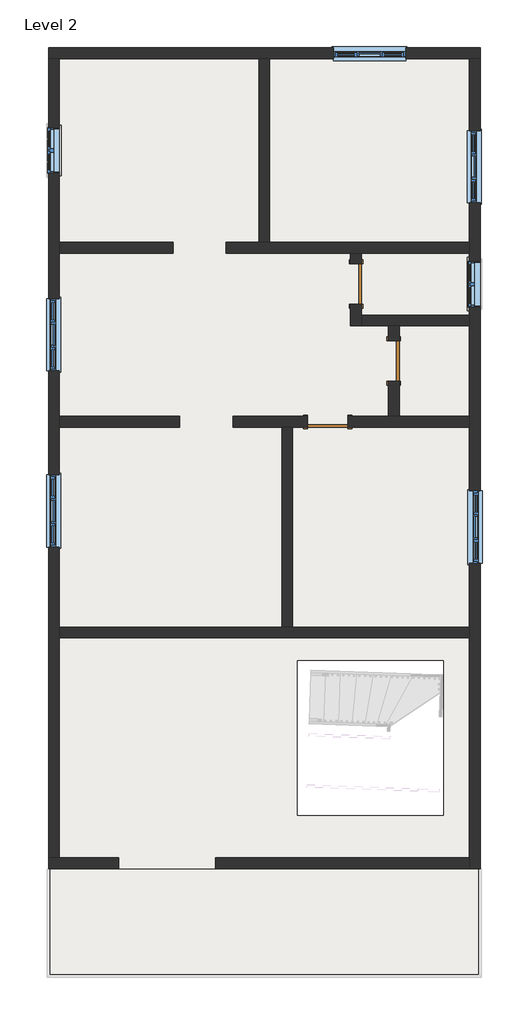
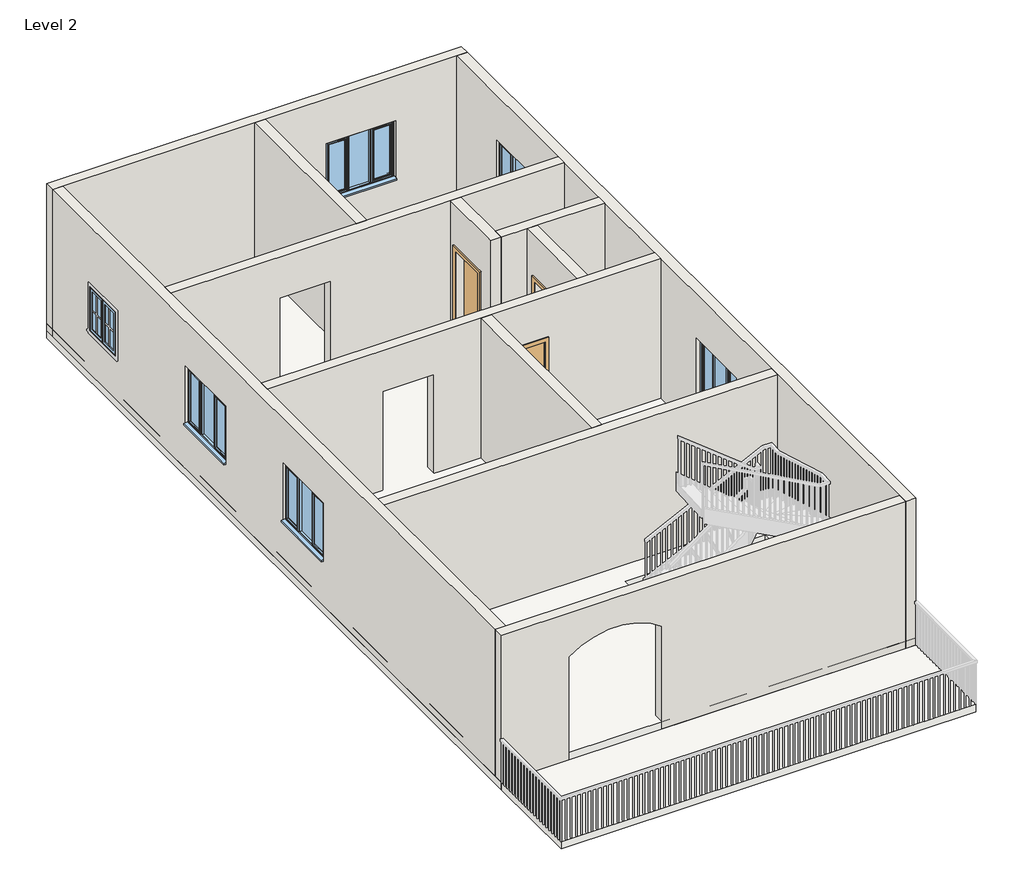
# One storey, part 1 of 3: 12 walls, 7 windows, 3 doors, 2 slabs, 1 roof.
"""IFC4 building model written with IfcOpenShell, lengths in millimetres."""

from ifc_helpers import new_model, si_unit, frame, origin, place, context, project, spatial, polyline, circle_curve, outline, extrude, faceted_brep, transform, mapped, element, save
from ifc_brep_helpers import plane_surface, revolved_surface, advanced_brep
from components import door_b6acaa4e, window_c29befe5, windows_tpl_plain_1360x1210mm_e2a6c9d8

model = new_model("IFC4")

# Units and contexts
model_context = context("Model", 3, world=origin())
ifc_project = project(units=[si_unit("LENGTHUNIT", "METRE", prefix="MILLI")], contexts=[model_context])

# Site, building, storey
site = spatial("IfcSite", under=ifc_project)
building = spatial("IfcBuilding", under=site)
storey = spatial("IfcBuildingStorey", under=building, Name="Level 2", Elevation=3048.0)

# Doors
placement = place(None, origin())
door_shape = door_b6acaa4e(model_context)
element("IfcDoor", 1, ObjectType="Single-Flush : 30\" x 84\"", at=placement, inside=storey, context=model_context, shape_type="MappedRepresentation", body=[
    mapped(door_shape, transform((-9158.3126504, 6947.728857, 3048.0), x_axis=(0.0, -1.0, 0.0), y_axis=(1.0, 0.0, 0.0), z_axis=(0.0, 0.0, 1.0))),
])
element("IfcDoor", 2, ObjectType="Single-Flush : 30\" x 84\"", at=placement, inside=storey, context=model_context, shape_type="MappedRepresentation", body=[
    mapped(door_shape, transform((-9691.7126504, 4356.928857, 3048.0), x_axis=(-1.0, 0.0, 0.0), y_axis=(0.0, -1.0, 0.0), z_axis=(0.0, 0.0, 1.0))),
])
element("IfcDoor", 3, ObjectType="Single-Flush : 30\" x 84\"", at=placement, inside=storey, context=model_context, shape_type="MappedRepresentation", body=[
    mapped(door_shape, transform((-8447.1126504, 5499.928857, 3048.0), x_axis=(0.0, -1.0, 0.0), y_axis=(1.0, 0.0, 0.0), z_axis=(0.0, 0.0, 1.0))),
])

# Roof
element("IfcRoof", 4, ObjectType="Generic - 12\"", at=placement, inside=storey, context=model_context, shape_type="SweptSolid", body=[
    extrude(outline(polyline([(-6821.5126504, 11392.728857), (-6821.5126504, -4050.471143), (-14949.5126504, -4050.471143), (-14949.5126504, 11392.728857), (-6821.5126504, 11392.728857)]), holes=[polyline([(-7518.4, -135.4836), (-10261.6, -135.4836), (-10261.6, -3048.381), (-7518.4, -3048.381), (-7518.4, -135.4836)])]), frame((0.0, 0.0, 3048.0), z_axis=(0.0, 0.0, 1.0), x_axis=(1.0, 0.0, 0.0)), (0.0, 0.0, 1.0), 152.4),
])

# Slabs
element("IfcSlab", 5, ObjectType="Generic - 12\"", at=placement, inside=storey, context=model_context, shape_type="SweptSolid", body=[
    extrude(outline(polyline([(-6821.5126504, 11392.728857), (-6821.5126504, -4050.471143), (-14949.5126504, -4050.471143), (-14949.5126504, 11392.728857), (-6821.5126504, 11392.728857)]), holes=[polyline([(-7518.4, -135.4836), (-10261.6, -135.4836), (-10261.6, -3048.381), (-7518.4, -3048.381), (-7518.4, -135.4836)])]), frame((0.0, 0.0, 2895.6), z_axis=(0.0, 0.0, 1.0), x_axis=(1.0, 0.0, 0.0)), (0.0, 0.0, 1.0), 152.4),
])
element("IfcSlab", 6, ObjectType="Generic - 12\"", at=placement, inside=storey, context=model_context, shape_type="SweptSolid", body=[
    extrude(outline(polyline([(-6821.5126504, -4050.471143), (-6821.5126504, -6082.471143), (-14949.5126504, -6082.471143), (-14949.5126504, -4050.471143), (-6821.5126504, -4050.471143)])), frame((0.0, 0.0, 2895.6), z_axis=(0.0, 0.0, 1.0), x_axis=(1.0, 0.0, 0.0)), (0.0, 0.0, 1.0), 152.4),
])

# Walls
element("IfcWall", 7, ObjectType="Generic - 4.5\" p", at=placement, inside=storey, context=model_context, shape_type="SweptSolid", body=[
    extrude(outline(polyline([(-10987.1126504, 7735.128857), (-10987.1126504, 11189.528857), (-10783.9126504, 11189.528857), (-10783.9126504, 7735.128857), (-10987.1126504, 7735.128857)])), frame((0.0, 0.0, 3048.0), z_axis=(0.0, 0.0, 1.0), x_axis=(1.0, 0.0, 0.0)), (0.0, 0.0, 1.0), 3048.0),
])
element("IfcWall", 8, ObjectType="Generic - 4.5\" p", at=placement, inside=storey, context=model_context, shape_type="Brep", body=[
    faceted_brep([(-7024.7126504, 7735.128857, 3048.0), (-10783.9126504, 7735.128857, 3048.0), (-10987.1126504, 7735.128857, 3048.0), (-11604.7126504, 7735.128857, 3048.0), (-11604.7126504, 7735.128857, 5248.0), (-12604.7126504, 7735.128857, 5248.0), (-12604.7126504, 7735.128857, 3048.0), (-14746.3126504, 7735.128857, 3048.0), (-14746.3126504, 7735.128857, 6096.0), (-10987.1126504, 7735.128857, 6096.0), (-10783.9126504, 7735.128857, 6096.0), (-7024.7126504, 7735.128857, 6096.0), (-11604.7126504, 7531.928857, 5248.0), (-11604.7126504, 7531.928857, 3048.0), (-9259.9126504, 7531.928857, 3048.0), (-9056.7126504, 7531.928857, 3048.0), (-7024.7126504, 7531.928857, 3048.0), (-7024.7126504, 7531.928857, 6096.0), (-9056.7126504, 7531.928857, 6096.0), (-9259.9126504, 7531.928857, 6096.0), (-14746.3126504, 7531.928857, 6096.0), (-14746.3126504, 7531.928857, 3048.0), (-12604.7126504, 7531.928857, 3048.0), (-12604.7126504, 7531.928857, 5248.0)], [[[0, 1, 2, 3, 4, 5, 6, 7, 8, 9, 10, 11]], [[12, 13, 14, 15, 16, 17, 18, 19, 20, 21, 22, 23]], [[22, 21, 7, 6]], [[16, 15, 14, 13, 3, 2, 1, 0]], [[11, 10, 9, 8, 20, 19, 18, 17]], [[8, 7, 21, 20]], [[0, 11, 17, 16]], [[4, 3, 13, 12]], [[5, 4, 12, 23]], [[6, 5, 23, 22]]]),
])
element("IfcWall", 9, ObjectType="Generic - 4.5\" p", at=placement, inside=storey, context=model_context, shape_type="Brep", body=[
    faceted_brep([(-9259.9126504, 6566.728857, 5181.6), (-9259.9126504, 6566.728857, 3048.0), (-9259.9126504, 6160.328857, 3048.0), (-9259.9126504, 6160.328857, 6096.0), (-9259.9126504, 7531.928857, 6096.0), (-9259.9126504, 7531.928857, 3048.0), (-9259.9126504, 7328.728857, 3048.0), (-9259.9126504, 7328.728857, 5181.6), (-9056.7126504, 6160.328857, 3048.0), (-9056.7126504, 6363.528857, 3048.0), (-9056.7126504, 6566.728857, 3048.0), (-9056.7126504, 6566.728857, 5181.6), (-9056.7126504, 7328.728857, 5181.6), (-9056.7126504, 7328.728857, 3048.0), (-9056.7126504, 7531.928857, 3048.0), (-9056.7126504, 7531.928857, 6096.0), (-9056.7126504, 6363.528857, 6096.0), (-9056.7126504, 6160.328857, 6096.0)], [[[0, 1, 2, 3, 4, 5, 6, 7]], [[8, 9, 10, 11, 12, 13, 14, 15, 16, 17]], [[6, 5, 14, 13]], [[2, 1, 10, 9, 8]], [[4, 3, 17, 16, 15]], [[5, 4, 15, 14]], [[3, 2, 8, 17]], [[11, 10, 1, 0]], [[12, 11, 0, 7]], [[13, 12, 7, 6]]]),
])
element("IfcWall", 10, ObjectType="Generic - 4.5\" p", at=placement, inside=storey, context=model_context, shape_type="Brep", body=[
    faceted_brep([(-9056.7126504, 6160.328857, 3048.0), (-8548.7126504, 6160.328857, 3048.0), (-8345.5126504, 6160.328857, 3048.0), (-7024.7126504, 6160.328857, 3048.0), (-7024.7126504, 6160.328857, 6096.0), (-8345.5126504, 6160.328857, 6096.0), (-8548.7126504, 6160.328857, 6096.0), (-9056.7126504, 6160.328857, 6096.0), (-9056.7126504, 6363.528857, 3048.0), (-9056.7126504, 6363.528857, 6096.0), (-7024.7126504, 6363.528857, 6096.0), (-7024.7126504, 6363.528857, 3048.0)], [[[0, 1, 2, 3, 4, 5, 6, 7]], [[8, 9, 10, 11]], [[3, 2, 1, 0, 8, 11]], [[7, 6, 5, 4, 10, 9]], [[0, 7, 9, 8]], [[4, 3, 11, 10]]]),
])
element("IfcWall", 11, ObjectType="Generic - 4.5\" p", at=placement, inside=storey, context=model_context, shape_type="SweptSolid", body=[
    extrude(outline(polyline([(5118.928857, 5181.6), (5118.928857, 3048.0), (4458.528857, 3048.0), (4458.528857, 6096.0), (6160.328857, 6096.0), (6160.328857, 3048.0), (5880.928857, 3048.0), (5880.928857, 5181.6), (5118.928857, 5181.6)])), frame((-8548.7126504, 0.0, 0.0), z_axis=(1.0, 0.0, 0.0), x_axis=(0.0, 1.0, 0.0)), (0.0, 0.0, 1.0), 203.2),
])
element("IfcWall", 12, ObjectType="Generic - 4.5\" p", at=placement, inside=storey, context=model_context, shape_type="Brep", body=[
    faceted_brep([(-10072.7126504, 4458.528857, 5181.6), (-10072.7126504, 4458.528857, 3048.0), (-11477.7126504, 4458.528857, 3048.0), (-11477.7126504, 4458.528857, 5248.0), (-12477.7126504, 4458.528857, 5248.0), (-12477.7126504, 4458.528857, 3048.0), (-14746.3126504, 4458.528857, 3048.0), (-14746.3126504, 4458.528857, 6096.0), (-8548.7126504, 4458.528857, 6096.0), (-8345.5126504, 4458.528857, 6096.0), (-7024.7126504, 4458.528857, 6096.0), (-7024.7126504, 4458.528857, 3048.0), (-8345.5126504, 4458.528857, 3048.0), (-8548.7126504, 4458.528857, 3048.0), (-9310.7126504, 4458.528857, 3048.0), (-9310.7126504, 4458.528857, 5181.6), (-11477.7126504, 4255.328857, 3048.0), (-10555.3126504, 4255.328857, 3048.0), (-10352.1126504, 4255.328857, 3048.0), (-10072.7126504, 4255.328857, 3048.0), (-10072.7126504, 4255.328857, 5181.6), (-9310.7126504, 4255.328857, 5181.6), (-9310.7126504, 4255.328857, 3048.0), (-7024.7126504, 4255.328857, 3048.0), (-7024.7126504, 4255.328857, 6096.0), (-10352.1126504, 4255.328857, 6096.0), (-10555.3126504, 4255.328857, 6096.0), (-14746.3126504, 4255.328857, 6096.0), (-14746.3126504, 4255.328857, 3048.0), (-12477.7126504, 4255.328857, 3048.0), (-12477.7126504, 4255.328857, 5248.0), (-11477.7126504, 4255.328857, 5248.0)], [[[0, 1, 2, 3, 4, 5, 6, 7, 8, 9, 10, 11, 12, 13, 14, 15]], [[16, 17, 18, 19, 20, 21, 22, 23, 24, 25, 26, 27, 28, 29, 30, 31]], [[29, 28, 6, 5]], [[2, 1, 19, 18, 17, 16]], [[14, 13, 12, 11, 23, 22]], [[10, 9, 8, 7, 27, 26, 25, 24]], [[11, 10, 24, 23]], [[7, 6, 28, 27]], [[3, 2, 16, 31]], [[4, 3, 31, 30]], [[5, 4, 30, 29]], [[20, 19, 1, 0]], [[21, 20, 0, 15]], [[22, 21, 15, 14]]]),
])
element("IfcWall", 13, ObjectType="Generic - 4.5\" p", at=placement, inside=storey, context=model_context, shape_type="SweptSolid", body=[
    extrude(outline(polyline([(-10555.3126504, 496.128857), (-10555.3126504, 4255.328857), (-10352.1126504, 4255.328857), (-10352.1126504, 496.128857), (-10555.3126504, 496.128857)])), frame((0.0, 0.0, 3048.0), z_axis=(0.0, 0.0, 1.0), x_axis=(1.0, 0.0, 0.0)), (0.0, 0.0, 1.0), 3048.0),
])
element("IfcWall", 14, ObjectType="Generic - 4.5\" p", at=placement, inside=storey, context=model_context, shape_type="Brep", body=[
    faceted_brep([(-14746.3126504, 292.928857, 3048.0), (-7024.7126504, 292.928857, 3048.0), (-7024.7126504, 292.928857, 6096.0), (-14746.3126504, 292.928857, 6096.0), (-14746.3126504, 496.128857, 3048.0), (-14746.3126504, 496.128857, 6096.0), (-10555.3126504, 496.128857, 6096.0), (-10352.1126504, 496.128857, 6096.0), (-7024.7126504, 496.128857, 6096.0), (-7024.7126504, 496.128857, 3048.0), (-10352.1126504, 496.128857, 3048.0), (-10555.3126504, 496.128857, 3048.0)], [[[0, 1, 2, 3]], [[4, 5, 6, 7, 8, 9, 10, 11]], [[1, 0, 4, 11, 10, 9]], [[3, 2, 8, 7, 6, 5]], [[2, 1, 9, 8]], [[0, 3, 5, 4]]]),
])
element("IfcWall", 15, ObjectType="Generic - 9\" w", at=placement, inside=storey, context=model_context, shape_type="Brep", body=[
    faceted_brep([(-14949.5126504, 11189.528857, 3048.0), (-14746.3126504, 11189.528857, 3048.0), (-10987.1126504, 11189.528857, 3048.0), (-10783.9126504, 11189.528857, 3048.0), (-7024.7126504, 11189.528857, 3048.0), (-6821.5126504, 11189.528857, 3048.0), (-6821.5126504, 11189.528857, 6096.0), (-7024.7126504, 11189.528857, 6096.0), (-10783.9126504, 11189.528857, 6096.0), (-10987.1126504, 11189.528857, 6096.0), (-14746.3126504, 11189.528857, 6096.0), (-14949.5126504, 11189.528857, 6096.0), (-8224.3126504, 11189.528857, 5172.4), (-8224.3126504, 11189.528857, 3962.4), (-9584.3126504, 11189.528857, 3962.4), (-9584.3126504, 11189.528857, 5172.4), (-14949.5126504, 11392.728857, 3048.0), (-14949.5126504, 11392.728857, 6096.0), (-6821.5126504, 11392.728857, 6096.0), (-6821.5126504, 11392.728857, 3048.0), (-8224.3126504, 11392.728857, 5172.4), (-9584.3126504, 11392.728857, 5172.4), (-9584.3126504, 11392.728857, 3962.4), (-8224.3126504, 11392.728857, 3962.4)], [[[0, 1, 2, 3, 4, 5, 6, 7, 8, 9, 10, 11], [12, 13, 14, 15]], [[16, 17, 18, 19], [20, 21, 22, 23]], [[5, 4, 3, 2, 1, 0, 16, 19]], [[11, 10, 9, 8, 7, 6, 18, 17]], [[6, 5, 19, 18]], [[0, 11, 17, 16]], [[13, 12, 20, 23]], [[14, 13, 23, 22]], [[15, 14, 22, 21]], [[12, 15, 21, 20]]]),
])
element("IfcWall", 16, ObjectType="Generic - 9\" w", at=placement, inside=storey, context=model_context, shape_type="Brep", body=[
    faceted_brep([(-7024.7126504, 11189.528857, 3048.0), (-7024.7126504, 7735.128857, 3048.0), (-7024.7126504, 7531.928857, 3048.0), (-7024.7126504, 6363.528857, 3048.0), (-7024.7126504, 6160.328857, 3048.0), (-7024.7126504, 4458.528857, 3048.0), (-7024.7126504, 4255.328857, 3048.0), (-7024.7126504, 496.128857, 3048.0), (-7024.7126504, 292.928857, 3048.0), (-7024.7126504, -3847.271143, 3048.0), (-7024.7126504, -4050.471143, 3048.0), (-7024.7126504, -4050.471143, 6096.0), (-7024.7126504, -3847.271143, 6096.0), (-7024.7126504, 292.928857, 6096.0), (-7024.7126504, 496.128857, 6096.0), (-7024.7126504, 4255.328857, 6096.0), (-7024.7126504, 4458.528857, 6096.0), (-7024.7126504, 6160.328857, 6096.0), (-7024.7126504, 6363.528857, 6096.0), (-7024.7126504, 7531.928857, 6096.0), (-7024.7126504, 7735.128857, 6096.0), (-7024.7126504, 11189.528857, 6096.0), (-7024.7126504, 8477.528857, 5172.4), (-7024.7126504, 8477.528857, 3962.4), (-7024.7126504, 9837.528857, 3962.4), (-7024.7126504, 9837.528857, 5172.4), (-7024.7126504, 3055.728857, 5172.4), (-7024.7126504, 1695.728857, 5172.4), (-7024.7126504, 1695.728857, 3962.4), (-7024.7126504, 3055.728857, 3962.4), (-7024.7126504, 7379.528857, 4876.8), (-7024.7126504, 6515.928857, 4876.8), (-7024.7126504, 6515.928857, 3962.4), (-7024.7126504, 7379.528857, 3962.4), (-6821.5126504, 11189.528857, 3048.0), (-6821.5126504, 11189.528857, 6096.0), (-6821.5126504, -4050.471143, 6096.0), (-6821.5126504, -4050.471143, 3048.0), (-6821.5126504, 8477.528857, 5172.4), (-6821.5126504, 9837.528857, 5172.4), (-6821.5126504, 9837.528857, 3962.4), (-6821.5126504, 8477.528857, 3962.4), (-6821.5126504, 3055.728857, 5172.4), (-6821.5126504, 3055.728857, 3962.4), (-6821.5126504, 1695.728857, 3962.4), (-6821.5126504, 1695.728857, 5172.4), (-6821.5126504, 7379.528857, 4876.8), (-6821.5126504, 7379.528857, 3962.4), (-6821.5126504, 6515.928857, 3962.4), (-6821.5126504, 6515.928857, 4876.8)], [[[0, 1, 2, 3, 4, 5, 6, 7, 8, 9, 10, 11, 12, 13, 14, 15, 16, 17, 18, 19, 20, 21], [22, 23, 24, 25], [26, 27, 28, 29], [30, 31, 32, 33]], [[34, 35, 36, 37], [38, 39, 40, 41], [42, 43, 44, 45], [46, 47, 48, 49]], [[10, 9, 8, 7, 6, 5, 4, 3, 2, 1, 0, 34, 37]], [[21, 20, 19, 18, 17, 16, 15, 14, 13, 12, 11, 36, 35]], [[0, 21, 35, 34]], [[11, 10, 37, 36]], [[23, 22, 38, 41]], [[24, 23, 41, 40]], [[25, 24, 40, 39]], [[22, 25, 39, 38]], [[43, 42, 26, 29]], [[44, 43, 29, 28]], [[45, 44, 28, 27]], [[42, 45, 27, 26]], [[47, 46, 30, 33]], [[48, 47, 33, 32]], [[49, 48, 32, 31]], [[46, 49, 31, 30]]]),
])
element("IfcWall", 17, ObjectType="Generic - 9\" w", at=placement, inside=storey, context=model_context, shape_type="AdvancedBrep", body=[
    advanced_brep(
    [(-14949.5126504, -3847.271143, 6096.0), (-14746.3126504, -3847.271143, 6096.0), (-7024.7126504, -3847.271143, 6096.0), (-7024.7126504, -3847.271143, 3048.0), (-11799.9126504, -3847.271143, 3048.0), (-11799.9126504, -3847.271143, 5181.6), (-13628.7126504, -3847.271143, 5181.6), (-13628.7126504, -3847.271143, 3048.0), (-14746.3126504, -3847.271143, 3048.0), (-14949.5126504, -3847.271143, 3048.0), (-7024.7126504, -4050.471143, 6096.0), (-14949.5126504, -4050.471143, 6096.0), (-14949.5126504, -4050.471143, 3048.0), (-13628.7126504, -4050.471143, 3048.0), (-13628.7126504, -4050.471143, 5181.6), (-11799.9126504, -4050.471143, 5181.6), (-11799.9126504, -4050.471143, 3048.0), (-7024.7126504, -4050.471143, 3048.0)],
    [
        (0, 1),
        (1, 2),
        (2, 3),
        (3, 4),
        (4, 5),
        (5, 6, circle_curve(frame((-12714.3126504, -3847.271143, 3965.0443508), z_axis=(0.0, -1.0, 0.0), x_axis=(1.0, 0.0, 0.0)), 1521.8853464)),
        (6, 7),
        (7, 8),
        (8, 9),
        (9, 0),
        (10, 11),
        (11, 12),
        (12, 13),
        (13, 14),
        (14, 15, circle_curve(frame((-12714.3126504, -4050.471143, 3965.0443508), z_axis=(0.0, 1.0, 0.0), x_axis=(1.0, 0.0, 0.0)), 1521.8853464)),
        (15, 16),
        (16, 17),
        (17, 10),
        (3, 17),
        (16, 4),
        (12, 9),
        (7, 13),
        (0, 11),
        (10, 2),
        (15, 5),
        (14, 6),
    ],
    [
        plane_surface(frame((-6923.1126504, -3847.271143, 3048.0), z_axis=(0.0, 1.0, 0.0), x_axis=(-1.0, 0.0, 0.0))),
        plane_surface(frame((-6923.1126504, -4050.471143, 3048.0), z_axis=(0.0, -1.0, 0.0), x_axis=(1.0, 0.0, 0.0))),
        plane_surface(frame((-6923.1126504, -3847.271143, 3048.0), z_axis=(0.0, 0.0, -1.0), x_axis=(0.0, -1.0, 0.0))),
        plane_surface(frame((-14847.9126504, -3847.271143, 6096.0), z_axis=(0.0, 0.0, 1.0), x_axis=(0.0, -1.0, 0.0))),
        plane_surface(frame((-7024.7126504, 11291.128857, 3048.0), z_axis=(1.0, 0.0, 0.0), x_axis=(0.0, -1.0, 0.0))),
        plane_surface(frame((-14949.5126504, -3948.871143, 3048.0), z_axis=(-1.0, 0.0, 0.0), x_axis=(0.0, -1.0, 0.0))),
        plane_surface(frame((-11799.9126504, -5574.471143, 3048.0), z_axis=(-1.0, 0.0, 0.0), x_axis=(0.0, 1.0, 0.0))),
        revolved_surface(polyline([(-11192.427303999999, -4050.471143, 3965.0443508), (-11192.427303999999, -3847.271143, 3965.0443508)]), (-12714.3126504, -2526.471143, 3965.0443508), (0.0, -1.0, 0.0)),
        plane_surface(frame((-13628.7126504, -5574.471143, 5181.6), z_axis=(1.0, 0.0, 0.0), x_axis=(0.0, 1.0, 0.0))),
    ],
    [
        (0, [[1, 2, 3, 4, 5, 6, 7, 8, 9, 10]]),
        (1, [[11, 12, 13, 14, 15, 16, 17, 18]]),
        (2, [[19, -17, 20, -4]]),
        (2, [[21, -9, -8, 22, -13]]),
        (3, [[-2, -1, 23, -11, 24]]),
        (4, [[-3, -24, -18, -19]]),
        (5, [[-10, -21, -12, -23]]),
        (6, [[25, -5, -20, -16]]),
        (7, [[-25, -15, 26, -6]]),
        (8, [[-26, -14, -22, -7]]),
    ],
),
])
element("IfcWall", 18, ObjectType="Generic - 9\" w", at=placement, inside=storey, context=model_context, shape_type="Brep", body=[
    faceted_brep([(-14746.3126504, -3847.271143, 3048.0), (-14746.3126504, 292.928857, 3048.0), (-14746.3126504, 496.128857, 3048.0), (-14746.3126504, 4255.328857, 3048.0), (-14746.3126504, 4458.528857, 3048.0), (-14746.3126504, 7531.928857, 3048.0), (-14746.3126504, 7735.128857, 3048.0), (-14746.3126504, 11189.528857, 3048.0), (-14746.3126504, 11189.528857, 6096.0), (-14746.3126504, 7735.128857, 6096.0), (-14746.3126504, 7531.928857, 6096.0), (-14746.3126504, 4458.528857, 6096.0), (-14746.3126504, 4255.328857, 6096.0), (-14746.3126504, 496.128857, 6096.0), (-14746.3126504, 292.928857, 6096.0), (-14746.3126504, -3847.271143, 6096.0), (-14746.3126504, 5315.228857, 5172.4), (-14746.3126504, 6675.228857, 5172.4), (-14746.3126504, 6675.228857, 3962.4), (-14746.3126504, 5315.228857, 3962.4), (-14746.3126504, 2000.528857, 5172.4), (-14746.3126504, 3360.528857, 5172.4), (-14746.3126504, 3360.528857, 3962.4), (-14746.3126504, 2000.528857, 3962.4), (-14746.3126504, 9894.128857, 4876.8), (-14746.3126504, 9894.128857, 3962.4), (-14746.3126504, 9030.528857, 3962.4), (-14746.3126504, 9030.528857, 4876.8), (-14949.5126504, -3847.271143, 3048.0), (-14949.5126504, -3847.271143, 6096.0), (-14949.5126504, 11189.528857, 6096.0), (-14949.5126504, 11189.528857, 3048.0), (-14949.5126504, 5315.228857, 5172.4), (-14949.5126504, 5315.228857, 3962.4), (-14949.5126504, 6675.228857, 3962.4), (-14949.5126504, 6675.228857, 5172.4), (-14949.5126504, 2000.528857, 5172.4), (-14949.5126504, 2000.528857, 3962.4), (-14949.5126504, 3360.528857, 3962.4), (-14949.5126504, 3360.528857, 5172.4), (-14949.5126504, 9894.128857, 4876.8), (-14949.5126504, 9030.528857, 4876.8), (-14949.5126504, 9030.528857, 3962.4), (-14949.5126504, 9894.128857, 3962.4)], [[[0, 1, 2, 3, 4, 5, 6, 7, 8, 9, 10, 11, 12, 13, 14, 15], [16, 17, 18, 19], [20, 21, 22, 23], [24, 25, 26, 27]], [[28, 29, 30, 31], [32, 33, 34, 35], [36, 37, 38, 39], [40, 41, 42, 43]], [[7, 6, 5, 4, 3, 2, 1, 0, 28, 31]], [[15, 14, 13, 12, 11, 10, 9, 8, 30, 29]], [[8, 7, 31, 30]], [[0, 15, 29, 28]], [[33, 32, 16, 19]], [[34, 33, 19, 18]], [[35, 34, 18, 17]], [[32, 35, 17, 16]], [[37, 36, 20, 23]], [[38, 37, 23, 22]], [[39, 38, 22, 21]], [[36, 39, 21, 20]], [[25, 24, 40, 43]], [[26, 25, 43, 42]], [[27, 26, 42, 41]], [[24, 27, 41, 40]]]),
])

# Windows
window_shape = window_c29befe5(model_context)
element("IfcWindow", 19, ObjectType="Window-Casement-Double : 34\" x 36\"", at=placement, inside=storey, context=model_context, shape_type="MappedRepresentation", body=[
    mapped(window_shape, transform((-14847.9126504, 9462.328857, 3048.0), x_axis=(0.0, 1.0, 0.0), y_axis=(-1.0, 0.0, 0.0), z_axis=(0.0, 0.0, 1.0))),
])
element("IfcWindow", 20, ObjectType="Window-Casement-Double : 34\" x 36\"", at=placement, inside=storey, context=model_context, shape_type="MappedRepresentation", body=[
    mapped(window_shape, transform((-6923.1126504, 6947.728857, 3048.0), x_axis=(0.0, 1.0, 0.0), y_axis=(-1.0, 0.0, 0.0), z_axis=(0.0, 0.0, 1.0))),
])
windows_tpl_plain_1360x1210mm_shape = windows_tpl_plain_1360x1210mm_e2a6c9d8(model_context)
element("IfcWindow", 21, ObjectType="Windows_Tpl_Plain : 1360x1210mm", at=placement, inside=storey, context=model_context, shape_type="MappedRepresentation", body=[
    mapped(windows_tpl_plain_1360x1210mm_shape, transform((-9405.979317, 11299.5854248, 3062.4), x_axis=(-1.0, 0.0, 0.0), y_axis=(0.0, -1.0, 0.0), z_axis=(0.0, 0.0, 1.0))),
])
element("IfcWindow", 22, ObjectType="Windows_Tpl_Plain : 1360x1210mm", at=placement, inside=storey, context=model_context, shape_type="MappedRepresentation", body=[
    mapped(windows_tpl_plain_1360x1210mm_shape, transform((-6914.6560825, 9659.1955236, 3062.4), x_axis=(0.0, 1.0, 0.0), y_axis=(-1.0, 0.0, 0.0), z_axis=(0.0, 0.0, 1.0))),
])
element("IfcWindow", 23, ObjectType="Windows_Tpl_Plain : 1360x1210mm", at=placement, inside=storey, context=model_context, shape_type="MappedRepresentation", body=[
    mapped(windows_tpl_plain_1360x1210mm_shape, transform((-6931.5692182, 1874.0621903, 3062.4), x_axis=(0.0, -1.0, 0.0), y_axis=(1.0, 0.0, 0.0), z_axis=(0.0, 0.0, 1.0))),
])
element("IfcWindow", 24, ObjectType="Windows_Tpl_Plain : 1360x1210mm", at=placement, inside=storey, context=model_context, shape_type="MappedRepresentation", body=[
    mapped(windows_tpl_plain_1360x1210mm_shape, transform((-14839.4560825, 6496.8955236, 3062.4), x_axis=(0.0, 1.0, 0.0), y_axis=(-1.0, 0.0, 0.0), z_axis=(0.0, 0.0, 1.0))),
])
element("IfcWindow", 25, ObjectType="Windows_Tpl_Plain : 1360x1210mm", at=placement, inside=storey, context=model_context, shape_type="MappedRepresentation", body=[
    mapped(windows_tpl_plain_1360x1210mm_shape, transform((-14839.4560825, 3182.1955236, 3062.4), x_axis=(0.0, 1.0, 0.0), y_axis=(-1.0, 0.0, 0.0), z_axis=(0.0, 0.0, 1.0))),
])

save(model, "model.ifc")

# Revit data of these elements
# Type "Single-Flush : 30\" x 84\""
#   Type Mark = "4"
#   Construction Type Id = "MDOOR"
#   Assembly Code = "C1020"
#   Analytic Construction = "Metal"
#   Thickness = 0' - 2"
#   Heat Transfer Coefficient (U) = 0.651978 BTU/(h·ft²·°F)
#   Height = 7' - 0"
#   Trim Projection Ext = 0' - 1"
#   Trim Projection Int = 0' - 1"
#   Trim Width = 0' - 3"
#   Width = 2' - 6"
#   Define Thermal Properties by = 1
#   Define Thermal Properties by = 1
#   Door Material = Door - Panel
#   Frame Material = Door - Frame
#   Visual Light Transmittance = 0
#   Solar Heat Gain Coefficient = 0
#   Function = (empty or 0)
#   Wall Closure = (empty or 0)
# Type "Generic - 12\""
#   Assembly Code = "B1020"
#   Layers, outside or top first: 0' - 6" no material (function 1)
# Type "Generic - 12\""
#   Assembly Code = "B1010"
#   Function = 0
#   Layers, outside or top first: 0' - 6" no material (function 1)
# Type "Generic - 4.5\" p"
#   Assembly Code = "B2010"
#   Layers, outside or top first: 0' - 8" "Brick, Common" (function 1)
# Type "Generic - 9\" w"
#   Assembly Code = "B2010"
#   Layers, outside or top first: 0' - 8" no material (function 1)
# Type "Window-Casement-Double : 34\" x 36\""
#   Type Mark = "14"
#   Fire Rating = "0.5h"
#   Assembly Code = "B2020100"
#   Analytic Construction = "Double glazing - domestic"
#   Frame Extension [instance default] = 0' - 0 1/4"
#   Window Inset [instance default] = 0' - 0"
#   Wall Thickness [instance default] = 0' - 6"
#   Interior Wall Closure [instance default] = 0' - 2 1/4"
#   Half Width = 1' - 5"
#   Visual Light Transmittance = 0.81
#   Thermal Resistance (R) = 1.8146 (h·ft²·°F)/BTU
#   Solar Heat Gain Coefficient = 0.76
#   Rough Width = 2' - 10 1/2"
#   Rough Height = 3' - 0 1/2"
#   Height = 3' - 0"
#   Heat Transfer Coefficient (U) = 0.5511 BTU/(h·ft²·°F)
#   Exterior Wall Closure [instance default] = 0' - 1 1/4"
#   Extension Jamb [instance default] = 0' - 2 1/4"
#   Default Sill Height = 3' - 0"
#   Width = 2' - 10"
#   Define Thermal Properties by = 0
#   Muntin Visibility = yes
#   Interior Trim Visibility [instance default] = yes
#   Exterior Trim Visibility [instance default] = yes
#   Extension Jamb Visibility [instance default] = yes
#   Interior Trim Material = Wood - Stained
#   Muntin Pattern = Muntin Pattern_2x2 : Muntin Pattern_2x2
#   Interior Trim = Trim-Window-Interior-Flat : Picture Frame
#   Interior Frame Material = Wood - Stained
#   Glass Panel Material = Glass
#   Exterior Trim Material = Clad - White
#   Exterior Trim = Trim-Window-Exterior-Flat : with Sill
#   Exterior Frame Material = Clad - White
#   Wall Closure = (empty or 0)
# Type "Windows_Tpl_Plain : 1360x1210mm"
#   Type Mark = "21"
#   Operation = "TriplePanelVertical"
#   Construction Type Id = "GSP4R"
#   Manufacturer = "Revit"
#   Keynote = "L10"
#   Analytic Construction = "1/8 in Pilkington single glazing"
#   Wrap Layers (Ext) from Ext = 0' - 4.03543"
#   Wrap Layers (Int) from Ext = 0' - 6.98819"
#   Window Board Projection = 0' - 0.98425"
#   Window Board Extension = 0' - 0.98425"
#   Visual Light Transmittance = 0.9
#   Solar Heat Gain Coefficient = 0.78
#   Rough Width = 4' - 5.54331"
#   Rough Height = 3' - 11.6378"
#   Height = 3' - 11.6378"
#   Width = 4' - 5.54331"
#   Heat Transfer Coefficient (U) = 0.6496 BTU/(h·ft²·°F)
#   Glazing Thickness = 0' - 0.94488"
#   FrameOffset - External = 0' - 1.9685"
#   Frame Depth = 0' - 2.55906"
#   Default Head Height = 6' - 11.07087"
#   Cill Depth = 0' - 3.44488"
#   Cavity Closer Width = 0' - 1.9685"
#   Cavity Closer Offset from Ext = 0' - 4.03543"
#   Cavity Closer Depth = 0' - 3.34646"
#   Vis - Cavity Closers = yes
#   Define Thermal Properties by = 1
#   Material Trim = Window Frame
#   Material Glass = Glass
#   Material Frame = Window Frame
#   Wall Closure = (empty or 0)
# Elements 1, 2, 3 (IfcDoor, "Single-Flush : 30\" x 84\"")
#   Phase Created = New Construction
#   Materials on its faces: "Door - Frame", "Door - Panel"
# Element 4 (IfcRoof, "Generic - 12\"")
#   built-in parameter 1001705 = 10.5 (stored number, unit not read)
#   built-in parameter 1001710 = 33615
#   Phase Created = New Construction
#   Materials on its faces: "Default Roof"
# Element 5 (IfcSlab, "Generic - 12\"")
#   Height Offset From Level = 0' - 0"
#   Phase Created = New Construction
#   Materials on its faces: "Default Floor", "Brick, Common"
# Element 6 (IfcSlab, "Generic - 12\"")
#   Height Offset From Level = 0' - 0"
#   Phase Created = New Construction
#   Materials on its faces: "Default Floor", "Analytical Floor Surface", "Brick, Soldier Course", "Concrete, Cast-in-Place gray"
# Elements 7, 8, 9, 11, 12, 13 (IfcWall, "Generic - 4.5\" p")
#   Top Offset = 0' - 0"
#   Base Offset = 0' - 0"
#   wall height = 10' - 0"
#   Phase Created = New Construction
#   Base Constraint = Level 2
#   Top Constraint = Level 3
#   Materials on its faces: "Brick, Common", "Cherry"
# Elements 10, 14 (IfcWall, "Generic - 4.5\" p")
#   Top Offset = 0' - 0"
#   Base Offset = 0' - 0"
#   wall height = 10' - 0"
#   Phase Created = New Construction
#   Base Constraint = Level 2
#   Top Constraint = Level 3
#   Materials on its faces: "Brick, Common"
# Elements 15, 18 (IfcWall, "Generic - 9\" w")
#   Top Offset = 0' - 0"
#   Base Offset = 0' - 0"
#   wall height = 10' - 0"
#   Phase Created = New Construction
#   Base Constraint = Level 2
#   Top Constraint = Level 3
#   Materials on its faces: "Default Wall", "Cherry"
# Element 16 (IfcWall, "Generic - 9\" w")
#   Top Offset = 0' - 0"
#   Base Offset = 0' - 0"
#   wall height = 10' - 0"
#   Phase Created = New Construction
#   Base Constraint = Level 2
#   Top Constraint = Level 3
#   Materials on its faces: "Default Wall", "Cherry", "Brick, Common"
# Element 17 (IfcWall, "Generic - 9\" w")
#   Top Offset = 0' - 0"
#   Base Offset = 0' - 0"
#   wall height = 10' - 0"
#   Phase Created = New Construction
#   Base Constraint = Level 2
#   Top Constraint = Level 3
#   Materials on its faces: "Default Wall", "Brick, Common"
# Element 19 (IfcWindow, "Window-Casement-Double : 34\" x 36\"")
#   Mark = "27"
#   Window Inset = 0' - 0"
#   Interior Wall Closure = 0' - 2 1/4"
#   Frame Extension = 0' - 0 1/4"
#   Exterior Wall Closure = 0' - 1 1/4"
#   Interior Trim Visibility = yes
#   Exterior Trim Visibility = yes
#   Phase Created = New Construction
#   Materials on its faces: "Wood - Stained", "Glass", "Clad - White"
# Element 20 (IfcWindow, "Window-Casement-Double : 34\" x 36\"")
#   Mark = "28"
#   Window Inset = 0' - 0"
#   Interior Wall Closure = 0' - 2 1/4"
#   Frame Extension = 0' - 0 1/4"
#   Exterior Wall Closure = 0' - 1 1/4"
#   Interior Trim Visibility = yes
#   Exterior Trim Visibility = yes
#   Phase Created = New Construction
#   Materials on its faces: "Wood - Stained", "Glass", "Clad - White"
# Element 21 (IfcWindow, "Windows_Tpl_Plain : 1360x1210mm")
#   Mark = "22"
#   Phase Created = New Construction
#   Materials on its faces: "Window Frame", "Glass"
# Element 22 (IfcWindow, "Windows_Tpl_Plain : 1360x1210mm")
#   Mark = "23"
#   Phase Created = New Construction
#   Materials on its faces: "Window Frame", "Glass"
# Element 23 (IfcWindow, "Windows_Tpl_Plain : 1360x1210mm")
#   Mark = "24"
#   Phase Created = New Construction
#   Materials on its faces: "Window Frame", "Glass"
# Element 24 (IfcWindow, "Windows_Tpl_Plain : 1360x1210mm")
#   Mark = "25"
#   Phase Created = New Construction
#   Materials on its faces: "Window Frame", "Glass"
# Element 25 (IfcWindow, "Windows_Tpl_Plain : 1360x1210mm")
#   Mark = "26"
#   Phase Created = New Construction
#   Materials on its faces: "Window Frame", "Glass"
# Materials
#   "Door - Panel": class "Wood", colour RGB 210 159 95, transparency 0, Cost = 0
#   "Door - Frame": colour RGB 118 70 51, transparency 0, Cost = 0
#   "Brick, Common": class "Masonry", colour RGB 128 0 128, transparency 0, Description = "Common brick", Cost = 0
#   "Wood - Stained": class "Wood", colour RGB 224 178 126, transparency 0, Cost = 0
#   "Glass": class "Glass", colour RGB 0 128 192, transparency 0.75, Description = "Soda Lime Glass", Cost = 0
#   "Clad - White": class "Wood", colour RGB 242 242 238, transparency 0, Cost = 0
#   "Window Frame": colour RGB 249 249 249, transparency 0
#   "Default Roof": colour RGB 88 101 114, transparency 0, Cost = 0
#   "Default Floor": colour RGB 128 128 128, transparency 0, Cost = 0
#   "Analytical Floor Surface": class "Generic", colour RGB 128 64 0, transparency 0.5, Cost = 0
#   "Brick, Soldier Course": class "Masonry", colour RGB 170 98 104, transparency 0, Description = "Common brick soldier coursed", Cost = 0
#   "Concrete, Cast-in-Place gray": class "Concrete", colour RGB 192 192 192, transparency 0, Description = "Cast-in-place concrete", Cost = 0
#   "Cherry": class "Wood", colour RGB 226 177 128, transparency 0, Description = "Prunus Serotina", Cost = 0
#   "Default Wall": colour RGB 128 128 128, transparency 0, Cost = 0
